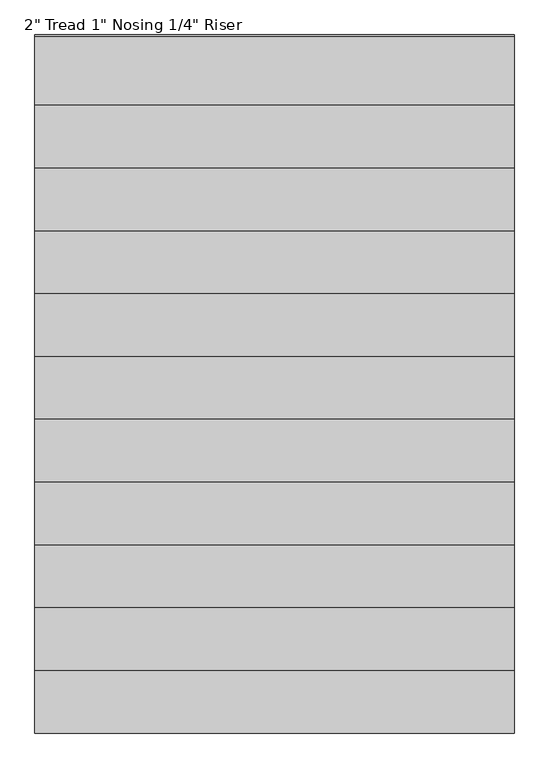
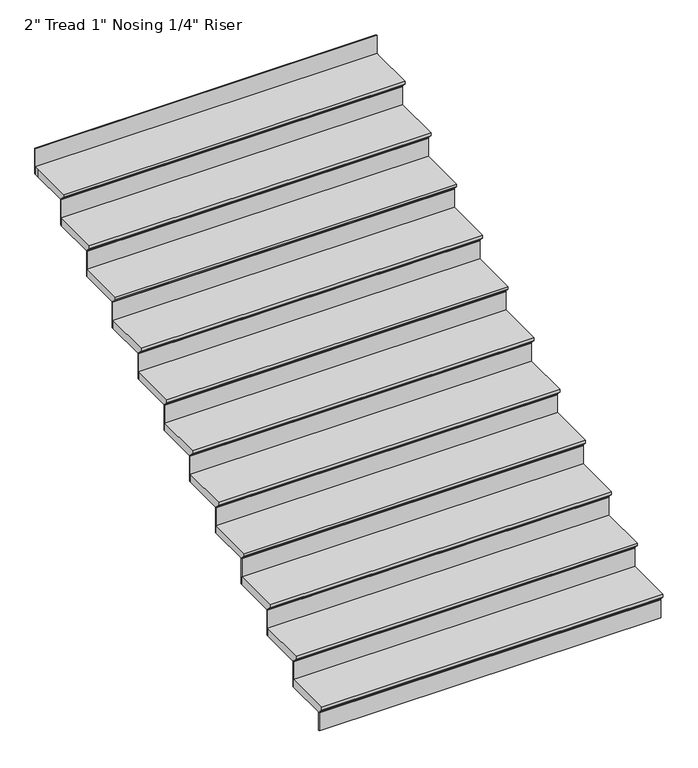
"""IFC4 building model written with IfcOpenShell, lengths in millimetres: stair flight geometry."""

from ifc_helpers import new_model, si_unit, origin, place, context, project, spatial, faceted_brep, source, transform, mapped, element, save


def stair_flight_3e597512(model_context):
    return source(origin(), model_context, "Body", "Brep", [
        faceted_brep([(-17843.6480019, -193.7741123, 150.2833333), (-17843.6480019, -193.7741123, 169.3333333), (-19977.2480019, -193.7741123, 169.3333333), (-19977.2480019, -193.7741123, 150.2833333), (-17843.6480019, -168.3741123, 124.8833333), (-19977.2480019, -168.3741123, 124.8833333), (-17843.6480019, 111.0258877, 169.3333333), (-19977.2480019, 111.0258877, 169.3333333), (-19977.2480019, -168.3741123, 118.5333333), (-19977.2480019, 111.0258877, 118.5333333), (-17843.6480019, 111.0258877, 118.5333333), (-17843.6480019, -168.3741123, 118.5333333)], [[[0, 1, 2, 3]], [[4, 0, 3, 5]], [[2, 1, 6, 7]], [[8, 9, 10, 11]], [[2, 7, 9, 8, 5, 3]], [[8, 11, 4, 5]], [[6, 1, 0, 4, 11, 10]], [[7, 6, 10, 9]]]),
        faceted_brep([(-17843.6480019, -168.3741123, 118.5333333), (-17843.6480019, -168.3741123, 0.0), (-17843.6480019, -162.0241123, 0.0), (-17843.6480019, -162.0241123, 118.5333333), (-19977.2480019, -168.3741123, 118.5333333), (-19977.2480019, -162.0241123, 118.5333333), (-19977.2480019, -162.0241123, 0.0), (-19977.2480019, -168.3741123, 0.0)], [[[0, 1, 2, 3]], [[4, 5, 6, 7]], [[1, 0, 4, 7]], [[2, 1, 7, 6]], [[3, 2, 6, 5]], [[0, 3, 5, 4]]]),
        faceted_brep([(-17843.6480019, 111.0258877, 287.8666667), (-17843.6480019, 111.0258877, 118.5333333), (-17843.6480019, 117.3758877, 118.5333333), (-17843.6480019, 117.3758877, 287.8666667), (-19977.2480019, 111.0258877, 287.8666667), (-19977.2480019, 117.3758877, 287.8666667), (-19977.2480019, 117.3758877, 118.5333333), (-19977.2480019, 111.0258877, 118.5333333)], [[[0, 1, 2, 3]], [[4, 5, 6, 7]], [[1, 0, 4, 7]], [[2, 1, 7, 6]], [[3, 2, 6, 5]], [[0, 3, 5, 4]]]),
        faceted_brep([(-19977.2480019, 85.6258877, 338.6666667), (-17843.6480019, 85.6258877, 338.6666667), (-17843.6480019, 390.4258877, 338.6666667), (-19977.2480019, 390.4258877, 338.6666667), (-19977.2480019, 111.0258877, 287.8666667), (-19977.2480019, 390.4258877, 287.8666667), (-17843.6480019, 390.4258877, 287.8666667), (-17843.6480019, 111.0258877, 287.8666667), (-19977.2480019, 111.0258877, 294.2166667), (-19977.2480019, 85.6258877, 319.6166667), (-17843.6480019, 111.0258877, 294.2166667), (-17843.6480019, 85.6258877, 319.6166667)], [[[0, 1, 2, 3]], [[4, 5, 6, 7]], [[0, 3, 5, 4, 8, 9]], [[4, 7, 10, 8]], [[2, 1, 11, 10, 7, 6]], [[3, 2, 6, 5]], [[11, 1, 0, 9]], [[10, 11, 9, 8]]]),
        faceted_brep([(-17843.6480019, 390.4258877, 457.2), (-17843.6480019, 390.4258877, 287.8666667), (-17843.6480019, 396.7758877, 287.8666667), (-17843.6480019, 396.7758877, 457.2), (-19977.2480019, 390.4258877, 457.2), (-19977.2480019, 396.7758877, 457.2), (-19977.2480019, 396.7758877, 287.8666667), (-19977.2480019, 390.4258877, 287.8666667)], [[[0, 1, 2, 3]], [[4, 5, 6, 7]], [[1, 0, 4, 7]], [[2, 1, 7, 6]], [[3, 2, 6, 5]], [[0, 3, 5, 4]]]),
        faceted_brep([(-19977.2480019, 365.0258877, 508.0), (-17843.6480019, 365.0258877, 508.0), (-17843.6480019, 669.8258877, 508.0), (-19977.2480019, 669.8258877, 508.0), (-19977.2480019, 390.4258877, 457.2), (-19977.2480019, 669.8258877, 457.2), (-17843.6480019, 669.8258877, 457.2), (-17843.6480019, 390.4258877, 457.2), (-19977.2480019, 390.4258877, 463.55), (-19977.2480019, 365.0258877, 488.95), (-17843.6480019, 390.4258877, 463.55), (-17843.6480019, 365.0258877, 488.95)], [[[0, 1, 2, 3]], [[4, 5, 6, 7]], [[0, 3, 5, 4, 8, 9]], [[4, 7, 10, 8]], [[2, 1, 11, 10, 7, 6]], [[3, 2, 6, 5]], [[11, 1, 0, 9]], [[10, 11, 9, 8]]]),
        faceted_brep([(-17843.6480019, 669.8258877, 626.5333333), (-17843.6480019, 669.8258877, 457.2), (-17843.6480019, 676.1758877, 457.2), (-17843.6480019, 676.1758877, 626.5333333), (-19977.2480019, 669.8258877, 626.5333333), (-19977.2480019, 676.1758877, 626.5333333), (-19977.2480019, 676.1758877, 457.2), (-19977.2480019, 669.8258877, 457.2)], [[[0, 1, 2, 3]], [[4, 5, 6, 7]], [[1, 0, 4, 7]], [[2, 1, 7, 6]], [[3, 2, 6, 5]], [[0, 3, 5, 4]]]),
        faceted_brep([(-19977.2480019, 644.4258877, 677.3333333), (-17843.6480019, 644.4258877, 677.3333333), (-17843.6480019, 949.2258877, 677.3333333), (-19977.2480019, 949.2258877, 677.3333333), (-19977.2480019, 669.8258877, 626.5333333), (-19977.2480019, 949.2258877, 626.5333333), (-17843.6480019, 949.2258877, 626.5333333), (-17843.6480019, 669.8258877, 626.5333333), (-19977.2480019, 669.8258877, 632.8833333), (-19977.2480019, 644.4258877, 658.2833333), (-17843.6480019, 669.8258877, 632.8833333), (-17843.6480019, 644.4258877, 658.2833333)], [[[0, 1, 2, 3]], [[4, 5, 6, 7]], [[0, 3, 5, 4, 8, 9]], [[4, 7, 10, 8]], [[2, 1, 11, 10, 7, 6]], [[3, 2, 6, 5]], [[11, 1, 0, 9]], [[10, 11, 9, 8]]]),
        faceted_brep([(-17843.6480019, 949.2258877, 795.8666667), (-17843.6480019, 949.2258877, 626.5333333), (-17843.6480019, 955.5758877, 626.5333333), (-17843.6480019, 955.5758877, 795.8666667), (-19977.2480019, 949.2258877, 795.8666667), (-19977.2480019, 955.5758877, 795.8666667), (-19977.2480019, 955.5758877, 626.5333333), (-19977.2480019, 949.2258877, 626.5333333)], [[[0, 1, 2, 3]], [[4, 5, 6, 7]], [[1, 0, 4, 7]], [[2, 1, 7, 6]], [[3, 2, 6, 5]], [[0, 3, 5, 4]]]),
        faceted_brep([(-19977.2480019, 923.8258877, 846.6666667), (-17843.6480019, 923.8258877, 846.6666667), (-17843.6480019, 1228.6258877, 846.6666667), (-19977.2480019, 1228.6258877, 846.6666667), (-19977.2480019, 949.2258877, 795.8666667), (-19977.2480019, 1228.6258877, 795.8666667), (-17843.6480019, 1228.6258877, 795.8666667), (-17843.6480019, 949.2258877, 795.8666667), (-19977.2480019, 949.2258877, 802.2166667), (-19977.2480019, 923.8258877, 827.6166667), (-17843.6480019, 949.2258877, 802.2166667), (-17843.6480019, 923.8258877, 827.6166667)], [[[0, 1, 2, 3]], [[4, 5, 6, 7]], [[0, 3, 5, 4, 8, 9]], [[4, 7, 10, 8]], [[2, 1, 11, 10, 7, 6]], [[3, 2, 6, 5]], [[11, 1, 0, 9]], [[10, 11, 9, 8]]]),
        faceted_brep([(-17843.6480019, 1228.6258877, 965.2), (-17843.6480019, 1228.6258877, 795.8666667), (-17843.6480019, 1234.9758877, 795.8666667), (-17843.6480019, 1234.9758877, 965.2), (-19977.2480019, 1228.6258877, 965.2), (-19977.2480019, 1234.9758877, 965.2), (-19977.2480019, 1234.9758877, 795.8666667), (-19977.2480019, 1228.6258877, 795.8666667)], [[[0, 1, 2, 3]], [[4, 5, 6, 7]], [[1, 0, 4, 7]], [[2, 1, 7, 6]], [[3, 2, 6, 5]], [[0, 3, 5, 4]]]),
        faceted_brep([(-19977.2480019, 1203.2258877, 1016.0), (-17843.6480019, 1203.2258877, 1016.0), (-17843.6480019, 1508.0258877, 1016.0), (-19977.2480019, 1508.0258877, 1016.0), (-19977.2480019, 1228.6258877, 965.2), (-19977.2480019, 1508.0258877, 965.2), (-17843.6480019, 1508.0258877, 965.2), (-17843.6480019, 1228.6258877, 965.2), (-19977.2480019, 1228.6258877, 971.55), (-19977.2480019, 1203.2258877, 996.95), (-17843.6480019, 1228.6258877, 971.55), (-17843.6480019, 1203.2258877, 996.95)], [[[0, 1, 2, 3]], [[4, 5, 6, 7]], [[0, 3, 5, 4, 8, 9]], [[4, 7, 10, 8]], [[2, 1, 11, 10, 7, 6]], [[3, 2, 6, 5]], [[11, 1, 0, 9]], [[10, 11, 9, 8]]]),
        faceted_brep([(-17843.6480019, 1508.0258877, 1134.5333333), (-17843.6480019, 1508.0258877, 965.2), (-17843.6480019, 1514.3758877, 965.2), (-17843.6480019, 1514.3758877, 1134.5333333), (-19977.2480019, 1508.0258877, 1134.5333333), (-19977.2480019, 1514.3758877, 1134.5333333), (-19977.2480019, 1514.3758877, 965.2), (-19977.2480019, 1508.0258877, 965.2)], [[[0, 1, 2, 3]], [[4, 5, 6, 7]], [[1, 0, 4, 7]], [[2, 1, 7, 6]], [[3, 2, 6, 5]], [[0, 3, 5, 4]]]),
        faceted_brep([(-19977.2480019, 1482.6258877, 1185.3333333), (-17843.6480019, 1482.6258877, 1185.3333333), (-17843.6480019, 1787.4258877, 1185.3333333), (-19977.2480019, 1787.4258877, 1185.3333333), (-19977.2480019, 1508.0258877, 1134.5333333), (-19977.2480019, 1787.4258877, 1134.5333333), (-17843.6480019, 1787.4258877, 1134.5333333), (-17843.6480019, 1508.0258877, 1134.5333333), (-19977.2480019, 1508.0258877, 1140.8833333), (-19977.2480019, 1482.6258877, 1166.2833333), (-17843.6480019, 1508.0258877, 1140.8833333), (-17843.6480019, 1482.6258877, 1166.2833333)], [[[0, 1, 2, 3]], [[4, 5, 6, 7]], [[0, 3, 5, 4, 8, 9]], [[4, 7, 10, 8]], [[2, 1, 11, 10, 7, 6]], [[3, 2, 6, 5]], [[11, 1, 0, 9]], [[10, 11, 9, 8]]]),
        faceted_brep([(-17843.6480019, 1787.4258877, 1303.8666667), (-17843.6480019, 1787.4258877, 1134.5333333), (-17843.6480019, 1793.7758877, 1134.5333333), (-17843.6480019, 1793.7758877, 1303.8666667), (-19977.2480019, 1787.4258877, 1303.8666667), (-19977.2480019, 1793.7758877, 1303.8666667), (-19977.2480019, 1793.7758877, 1134.5333333), (-19977.2480019, 1787.4258877, 1134.5333333)], [[[0, 1, 2, 3]], [[4, 5, 6, 7]], [[1, 0, 4, 7]], [[2, 1, 7, 6]], [[3, 2, 6, 5]], [[0, 3, 5, 4]]]),
        faceted_brep([(-19977.2480019, 1762.0258877, 1354.6666667), (-17843.6480019, 1762.0258877, 1354.6666667), (-17843.6480019, 2066.8258877, 1354.6666667), (-19977.2480019, 2066.8258877, 1354.6666667), (-19977.2480019, 1787.4258877, 1303.8666667), (-19977.2480019, 2066.8258877, 1303.8666667), (-17843.6480019, 2066.8258877, 1303.8666667), (-17843.6480019, 1787.4258877, 1303.8666667), (-19977.2480019, 1787.4258877, 1310.2166667), (-19977.2480019, 1762.0258877, 1335.6166667), (-17843.6480019, 1787.4258877, 1310.2166667), (-17843.6480019, 1762.0258877, 1335.6166667)], [[[0, 1, 2, 3]], [[4, 5, 6, 7]], [[0, 3, 5, 4, 8, 9]], [[4, 7, 10, 8]], [[2, 1, 11, 10, 7, 6]], [[3, 2, 6, 5]], [[11, 1, 0, 9]], [[10, 11, 9, 8]]]),
        faceted_brep([(-17843.6480019, 2066.8258877, 1473.2), (-17843.6480019, 2066.8258877, 1303.8666667), (-17843.6480019, 2073.1758877, 1303.8666667), (-17843.6480019, 2073.1758877, 1473.2), (-19977.2480019, 2066.8258877, 1473.2), (-19977.2480019, 2073.1758877, 1473.2), (-19977.2480019, 2073.1758877, 1303.8666667), (-19977.2480019, 2066.8258877, 1303.8666667)], [[[0, 1, 2, 3]], [[4, 5, 6, 7]], [[1, 0, 4, 7]], [[2, 1, 7, 6]], [[3, 2, 6, 5]], [[0, 3, 5, 4]]]),
        faceted_brep([(-19977.2480019, 2041.4258877, 1524.0), (-17843.6480019, 2041.4258877, 1524.0), (-17843.6480019, 2346.2258877, 1524.0), (-19977.2480019, 2346.2258877, 1524.0), (-19977.2480019, 2066.8258877, 1473.2), (-19977.2480019, 2346.2258877, 1473.2), (-17843.6480019, 2346.2258877, 1473.2), (-17843.6480019, 2066.8258877, 1473.2), (-19977.2480019, 2066.8258877, 1479.55), (-19977.2480019, 2041.4258877, 1504.95), (-17843.6480019, 2066.8258877, 1479.55), (-17843.6480019, 2041.4258877, 1504.95)], [[[0, 1, 2, 3]], [[4, 5, 6, 7]], [[0, 3, 5, 4, 8, 9]], [[4, 7, 10, 8]], [[2, 1, 11, 10, 7, 6]], [[3, 2, 6, 5]], [[11, 1, 0, 9]], [[10, 11, 9, 8]]]),
        faceted_brep([(-17843.6480019, 2346.2258877, 1642.5333333), (-17843.6480019, 2346.2258877, 1473.2), (-17843.6480019, 2352.5758877, 1473.2), (-17843.6480019, 2352.5758877, 1642.5333333), (-19977.2480019, 2346.2258877, 1642.5333333), (-19977.2480019, 2352.5758877, 1642.5333333), (-19977.2480019, 2352.5758877, 1473.2), (-19977.2480019, 2346.2258877, 1473.2)], [[[0, 1, 2, 3]], [[4, 5, 6, 7]], [[1, 0, 4, 7]], [[2, 1, 7, 6]], [[3, 2, 6, 5]], [[0, 3, 5, 4]]]),
        faceted_brep([(-19977.2480019, 2320.8258877, 1693.3333333), (-17843.6480019, 2320.8258877, 1693.3333333), (-17843.6480019, 2625.6258877, 1693.3333333), (-19977.2480019, 2625.6258877, 1693.3333333), (-19977.2480019, 2346.2258877, 1642.5333333), (-19977.2480019, 2625.6258877, 1642.5333333), (-17843.6480019, 2625.6258877, 1642.5333333), (-17843.6480019, 2346.2258877, 1642.5333333), (-19977.2480019, 2346.2258877, 1648.8833333), (-19977.2480019, 2320.8258877, 1674.2833333), (-17843.6480019, 2346.2258877, 1648.8833333), (-17843.6480019, 2320.8258877, 1674.2833333)], [[[0, 1, 2, 3]], [[4, 5, 6, 7]], [[0, 3, 5, 4, 8, 9]], [[4, 7, 10, 8]], [[2, 1, 11, 10, 7, 6]], [[3, 2, 6, 5]], [[11, 1, 0, 9]], [[10, 11, 9, 8]]]),
        faceted_brep([(-17843.6480019, 2905.0258877, 1981.2), (-17843.6480019, 2905.0258877, 1811.8666667), (-17843.6480019, 2911.3758877, 1811.8666667), (-17843.6480019, 2911.3758877, 1981.2), (-19977.2480019, 2905.0258877, 1981.2), (-19977.2480019, 2911.3758877, 1981.2), (-19977.2480019, 2911.3758877, 1811.8666667), (-19977.2480019, 2905.0258877, 1811.8666667)], [[[0, 1, 2, 3]], [[4, 5, 6, 7]], [[1, 0, 4, 7]], [[2, 1, 7, 6]], [[3, 2, 6, 5]], [[0, 3, 5, 4]]]),
        faceted_brep([(-17843.6480019, 2625.6258877, 1811.8666667), (-17843.6480019, 2625.6258877, 1642.5333333), (-17843.6480019, 2631.9758877, 1642.5333333), (-17843.6480019, 2631.9758877, 1811.8666667), (-19977.2480019, 2625.6258877, 1811.8666667), (-19977.2480019, 2631.9758877, 1811.8666667), (-19977.2480019, 2631.9758877, 1642.5333333), (-19977.2480019, 2625.6258877, 1642.5333333)], [[[0, 1, 2, 3]], [[4, 5, 6, 7]], [[1, 0, 4, 7]], [[2, 1, 7, 6]], [[3, 2, 6, 5]], [[0, 3, 5, 4]]]),
        faceted_brep([(-19977.2480019, 2905.0258877, 1862.6666667), (-19977.2480019, 2879.6258877, 1862.6666667), (-19977.2480019, 2600.2258877, 1862.6666667), (-17843.6480019, 2600.2258877, 1862.6666667), (-17843.6480019, 2879.6258877, 1862.6666667), (-17843.6480019, 2905.0258877, 1862.6666667), (-19977.2480019, 2879.6258877, 1811.8666667), (-19977.2480019, 2905.0258877, 1811.8666667), (-17843.6480019, 2905.0258877, 1811.8666667), (-17843.6480019, 2879.6258877, 1811.8666667), (-17843.6480019, 2625.6258877, 1811.8666667), (-19977.2480019, 2625.6258877, 1811.8666667), (-19977.2480019, 2625.6258877, 1818.2166667), (-19977.2480019, 2600.2258877, 1843.6166667), (-17843.6480019, 2625.6258877, 1818.2166667), (-17843.6480019, 2600.2258877, 1843.6166667)], [[[0, 1, 2, 3, 4, 5]], [[6, 7, 8, 9, 10, 11]], [[1, 0, 7, 6]], [[2, 1, 6, 11, 12, 13]], [[11, 10, 14, 12]], [[4, 3, 15, 14, 10, 9]], [[0, 5, 8, 7]], [[15, 3, 2, 13]], [[14, 15, 13, 12]], [[5, 4, 9, 8]]]),
    ])


if __name__ == "__main__":
    model = new_model("IFC4")
    model_context = context("Model", 3, world=origin())
    ifc_project = project(units=[si_unit("LENGTHUNIT", "METRE", prefix="MILLI")], contexts=[model_context])
    site = spatial("IfcSite", under=ifc_project)
    building = spatial("IfcBuilding", under=site)
    placement = place(None, origin())
    stair_flight_shape = stair_flight_3e597512(model_context)
    element("IfcStairFlight", 1, ObjectType="2\" Tread 1\" Nosing 1/4\" Riser", at=placement, inside=building, context=model_context, shape_type="MappedRepresentation", body=[
        mapped(stair_flight_shape, transform((0.0, 0.0, 0.0), x_axis=(1.0, 0.0, 0.0), y_axis=(0.0, 1.0, 0.0), z_axis=(0.0, 0.0, 1.0))),
    ])
    save(model, "model.ifc")
